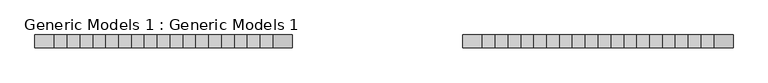
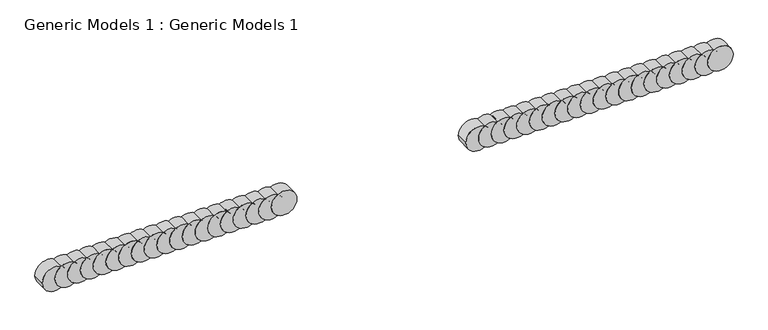
"""IFC4 building model written with IfcOpenShell, lengths in millimetres: proxy geometry, Generic Models 1 : Generic Models 1."""

from ifc_helpers import new_model, si_unit, point, frame, frame_2d, origin, place, context, project, spatial, circle_curve, trimmed, segment, composite_curve, outline, extrude, source, transform, mapped, element, save


def generic_models_1_generic_models_1_03ad02fd(model_context):
    return source(origin(), model_context, "Body", "SweptSolid", [
        extrude(outline(composite_curve([segment(trimmed(circle_curve(frame_2d((571.1323801, 6489.1161456)), 304.8), [point((571.1323801, 6184.3161456))], [point((571.1323801, 6793.9161456))], False, "CARTESIAN"), True, "CONTINUOUS"), segment(trimmed(circle_curve(frame_2d((571.1323801, 6489.1161456)), 304.8), [point((571.1323801, 6793.9161456))], [point((571.1323801, 6184.3161456))], False, "CARTESIAN"), True, "CONTINUOUS")], self_intersect=False)), frame((0.0, -13009.1052022, 0.0), z_axis=(0.0, 1.0, 0.0), x_axis=(0.0, 0.0, 1.0)), (0.0, 0.0, 1.0), 304.8),
        extrude(outline(composite_curve([segment(trimmed(circle_curve(frame_2d((571.1323801, 6184.3161456)), 304.8), [point((571.1323801, 5879.5161456))], [point((571.1323801, 6489.1161456))], False, "CARTESIAN"), True, "CONTINUOUS"), segment(trimmed(circle_curve(frame_2d((571.1323801, 6184.3161456)), 304.8), [point((571.1323801, 6489.1161456))], [point((571.1323801, 5879.5161456))], False, "CARTESIAN"), True, "CONTINUOUS")], self_intersect=False)), frame((0.0, -13009.1052022, 0.0), z_axis=(0.0, 1.0, 0.0), x_axis=(0.0, 0.0, 1.0)), (0.0, 0.0, 1.0), 304.8),
        extrude(outline(composite_curve([segment(trimmed(circle_curve(frame_2d((571.1323801, 5879.5161456)), 304.8), [point((571.1323801, 5574.7161456))], [point((571.1323801, 6184.3161456))], False, "CARTESIAN"), True, "CONTINUOUS"), segment(trimmed(circle_curve(frame_2d((571.1323801, 5879.5161456)), 304.8), [point((571.1323801, 6184.3161456))], [point((571.1323801, 5574.7161456))], False, "CARTESIAN"), True, "CONTINUOUS")], self_intersect=False)), frame((0.0, -13009.1052022, 0.0), z_axis=(0.0, 1.0, 0.0), x_axis=(0.0, 0.0, 1.0)), (0.0, 0.0, 1.0), 304.8),
        extrude(outline(composite_curve([segment(trimmed(circle_curve(frame_2d((571.1323801, 5574.7161456)), 304.8), [point((571.1323801, 5269.9161456))], [point((571.1323801, 5879.5161456))], False, "CARTESIAN"), True, "CONTINUOUS"), segment(trimmed(circle_curve(frame_2d((571.1323801, 5574.7161456)), 304.8), [point((571.1323801, 5879.5161456))], [point((571.1323801, 5269.9161456))], False, "CARTESIAN"), True, "CONTINUOUS")], self_intersect=False)), frame((0.0, -13009.1052022, 0.0), z_axis=(0.0, 1.0, 0.0), x_axis=(0.0, 0.0, 1.0)), (0.0, 0.0, 1.0), 304.8),
        extrude(outline(composite_curve([segment(trimmed(circle_curve(frame_2d((571.1323801, 5269.9161456)), 304.8), [point((571.1323801, 4965.1161456))], [point((571.1323801, 5574.7161456))], False, "CARTESIAN"), True, "CONTINUOUS"), segment(trimmed(circle_curve(frame_2d((571.1323801, 5269.9161456)), 304.8), [point((571.1323801, 5574.7161456))], [point((571.1323801, 4965.1161456))], False, "CARTESIAN"), True, "CONTINUOUS")], self_intersect=False)), frame((0.0, -13009.1052022, 0.0), z_axis=(0.0, 1.0, 0.0), x_axis=(0.0, 0.0, 1.0)), (0.0, 0.0, 1.0), 304.8),
        extrude(outline(composite_curve([segment(trimmed(circle_curve(frame_2d((571.1323801, 4965.1161456)), 304.8), [point((571.1323801, 4660.3161456))], [point((571.1323801, 5269.9161456))], False, "CARTESIAN"), True, "CONTINUOUS"), segment(trimmed(circle_curve(frame_2d((571.1323801, 4965.1161456)), 304.8), [point((571.1323801, 5269.9161456))], [point((571.1323801, 4660.3161456))], False, "CARTESIAN"), True, "CONTINUOUS")], self_intersect=False)), frame((0.0, -13009.1052022, 0.0), z_axis=(0.0, 1.0, 0.0), x_axis=(0.0, 0.0, 1.0)), (0.0, 0.0, 1.0), 304.8),
        extrude(outline(composite_curve([segment(trimmed(circle_curve(frame_2d((571.1323801, 4660.3161456)), 304.8), [point((571.1323801, 4355.5161456))], [point((571.1323801, 4965.1161456))], False, "CARTESIAN"), True, "CONTINUOUS"), segment(trimmed(circle_curve(frame_2d((571.1323801, 4660.3161456)), 304.8), [point((571.1323801, 4965.1161456))], [point((571.1323801, 4355.5161456))], False, "CARTESIAN"), True, "CONTINUOUS")], self_intersect=False)), frame((0.0, -13009.1052022, 0.0), z_axis=(0.0, 1.0, 0.0), x_axis=(0.0, 0.0, 1.0)), (0.0, 0.0, 1.0), 304.8),
        extrude(outline(composite_curve([segment(trimmed(circle_curve(frame_2d((571.1323801, 4355.5161456)), 304.8), [point((571.1323801, 4050.7161456))], [point((571.1323801, 4660.3161456))], False, "CARTESIAN"), True, "CONTINUOUS"), segment(trimmed(circle_curve(frame_2d((571.1323801, 4355.5161456)), 304.8), [point((571.1323801, 4660.3161456))], [point((571.1323801, 4050.7161456))], False, "CARTESIAN"), True, "CONTINUOUS")], self_intersect=False)), frame((0.0, -13009.1052022, 0.0), z_axis=(0.0, 1.0, 0.0), x_axis=(0.0, 0.0, 1.0)), (0.0, 0.0, 1.0), 304.8),
        extrude(outline(composite_curve([segment(trimmed(circle_curve(frame_2d((571.1323801, 4050.7161456)), 304.8), [point((571.1323801, 3745.9161456))], [point((571.1323801, 4355.5161456))], False, "CARTESIAN"), True, "CONTINUOUS"), segment(trimmed(circle_curve(frame_2d((571.1323801, 4050.7161456)), 304.8), [point((571.1323801, 4355.5161456))], [point((571.1323801, 3745.9161456))], False, "CARTESIAN"), True, "CONTINUOUS")], self_intersect=False)), frame((0.0, -13009.1052022, 0.0), z_axis=(0.0, 1.0, 0.0), x_axis=(0.0, 0.0, 1.0)), (0.0, 0.0, 1.0), 304.8),
        extrude(outline(composite_curve([segment(trimmed(circle_curve(frame_2d((571.1323801, 3745.9161456)), 304.8), [point((571.1323801, 3441.1161456))], [point((571.1323801, 4050.7161456))], False, "CARTESIAN"), True, "CONTINUOUS"), segment(trimmed(circle_curve(frame_2d((571.1323801, 3745.9161456)), 304.8), [point((571.1323801, 4050.7161456))], [point((571.1323801, 3441.1161456))], False, "CARTESIAN"), True, "CONTINUOUS")], self_intersect=False)), frame((0.0, -13009.1052022, 0.0), z_axis=(0.0, 1.0, 0.0), x_axis=(0.0, 0.0, 1.0)), (0.0, 0.0, 1.0), 304.8),
        extrude(outline(composite_curve([segment(trimmed(circle_curve(frame_2d((571.1323801, 3441.1161456)), 304.8), [point((571.1323801, 3136.3161456))], [point((571.1323801, 3745.9161456))], False, "CARTESIAN"), True, "CONTINUOUS"), segment(trimmed(circle_curve(frame_2d((571.1323801, 3441.1161456)), 304.8), [point((571.1323801, 3745.9161456))], [point((571.1323801, 3136.3161456))], False, "CARTESIAN"), True, "CONTINUOUS")], self_intersect=False)), frame((0.0, -13009.1052022, 0.0), z_axis=(0.0, 1.0, 0.0), x_axis=(0.0, 0.0, 1.0)), (0.0, 0.0, 1.0), 304.8),
        extrude(outline(composite_curve([segment(trimmed(circle_curve(frame_2d((571.1323801, 3136.3161456)), 304.8), [point((571.1323801, 2831.5161456))], [point((571.1323801, 3441.1161456))], False, "CARTESIAN"), True, "CONTINUOUS"), segment(trimmed(circle_curve(frame_2d((571.1323801, 3136.3161456)), 304.8), [point((571.1323801, 3441.1161456))], [point((571.1323801, 2831.5161456))], False, "CARTESIAN"), True, "CONTINUOUS")], self_intersect=False)), frame((0.0, -13009.1052022, 0.0), z_axis=(0.0, 1.0, 0.0), x_axis=(0.0, 0.0, 1.0)), (0.0, 0.0, 1.0), 304.8),
        extrude(outline(composite_curve([segment(trimmed(circle_curve(frame_2d((571.1323801, 2831.5161456)), 304.8), [point((571.1323801, 2526.7161456))], [point((571.1323801, 3136.3161456))], False, "CARTESIAN"), True, "CONTINUOUS"), segment(trimmed(circle_curve(frame_2d((571.1323801, 2831.5161456)), 304.8), [point((571.1323801, 3136.3161456))], [point((571.1323801, 2526.7161456))], False, "CARTESIAN"), True, "CONTINUOUS")], self_intersect=False)), frame((0.0, -13009.1052022, 0.0), z_axis=(0.0, 1.0, 0.0), x_axis=(0.0, 0.0, 1.0)), (0.0, 0.0, 1.0), 304.8),
        extrude(outline(composite_curve([segment(trimmed(circle_curve(frame_2d((571.1323801, 2526.7161456)), 304.8), [point((571.1323801, 2221.9161456))], [point((571.1323801, 2831.5161456))], False, "CARTESIAN"), True, "CONTINUOUS"), segment(trimmed(circle_curve(frame_2d((571.1323801, 2526.7161456)), 304.8), [point((571.1323801, 2831.5161456))], [point((571.1323801, 2221.9161456))], False, "CARTESIAN"), True, "CONTINUOUS")], self_intersect=False)), frame((0.0, -13009.1052022, 0.0), z_axis=(0.0, 1.0, 0.0), x_axis=(0.0, 0.0, 1.0)), (0.0, 0.0, 1.0), 304.8),
        extrude(outline(composite_curve([segment(trimmed(circle_curve(frame_2d((571.1323801, 2221.9161456)), 304.8), [point((571.1323801, 1917.1161456))], [point((571.1323801, 2526.7161456))], False, "CARTESIAN"), True, "CONTINUOUS"), segment(trimmed(circle_curve(frame_2d((571.1323801, 2221.9161456)), 304.8), [point((571.1323801, 2526.7161456))], [point((571.1323801, 1917.1161456))], False, "CARTESIAN"), True, "CONTINUOUS")], self_intersect=False)), frame((0.0, -13009.1052022, 0.0), z_axis=(0.0, 1.0, 0.0), x_axis=(0.0, 0.0, 1.0)), (0.0, 0.0, 1.0), 304.8),
        extrude(outline(composite_curve([segment(trimmed(circle_curve(frame_2d((571.1323801, 1917.1161456)), 304.8), [point((571.1323801, 1612.3161456))], [point((571.1323801, 2221.9161456))], False, "CARTESIAN"), True, "CONTINUOUS"), segment(trimmed(circle_curve(frame_2d((571.1323801, 1917.1161456)), 304.8), [point((571.1323801, 2221.9161456))], [point((571.1323801, 1612.3161456))], False, "CARTESIAN"), True, "CONTINUOUS")], self_intersect=False)), frame((0.0, -13009.1052022, 0.0), z_axis=(0.0, 1.0, 0.0), x_axis=(0.0, 0.0, 1.0)), (0.0, 0.0, 1.0), 304.8),
        extrude(outline(composite_curve([segment(trimmed(circle_curve(frame_2d((571.1323801, 1612.3161456)), 304.8), [point((571.1323801, 1307.5161456))], [point((571.1323801, 1917.1161456))], False, "CARTESIAN"), True, "CONTINUOUS"), segment(trimmed(circle_curve(frame_2d((571.1323801, 1612.3161456)), 304.8), [point((571.1323801, 1917.1161456))], [point((571.1323801, 1307.5161456))], False, "CARTESIAN"), True, "CONTINUOUS")], self_intersect=False)), frame((0.0, -13009.1052022, 0.0), z_axis=(0.0, 1.0, 0.0), x_axis=(0.0, 0.0, 1.0)), (0.0, 0.0, 1.0), 304.8),
        extrude(outline(composite_curve([segment(trimmed(circle_curve(frame_2d((571.1323801, 1307.5161456)), 304.8), [point((571.1323801, 1002.7161456))], [point((571.1323801, 1612.3161456))], False, "CARTESIAN"), True, "CONTINUOUS"), segment(trimmed(circle_curve(frame_2d((571.1323801, 1307.5161456)), 304.8), [point((571.1323801, 1612.3161456))], [point((571.1323801, 1002.7161456))], False, "CARTESIAN"), True, "CONTINUOUS")], self_intersect=False)), frame((0.0, -13009.1052022, 0.0), z_axis=(0.0, 1.0, 0.0), x_axis=(0.0, 0.0, 1.0)), (0.0, 0.0, 1.0), 304.8),
        extrude(outline(composite_curve([segment(trimmed(circle_curve(frame_2d((571.1323801, 1002.7161456)), 304.8), [point((571.1323801, 697.9161456))], [point((571.1323801, 1307.5161456))], False, "CARTESIAN"), True, "CONTINUOUS"), segment(trimmed(circle_curve(frame_2d((571.1323801, 1002.7161456)), 304.8), [point((571.1323801, 1307.5161456))], [point((571.1323801, 697.9161456))], False, "CARTESIAN"), True, "CONTINUOUS")], self_intersect=False)), frame((0.0, -13009.1052022, 0.0), z_axis=(0.0, 1.0, 0.0), x_axis=(0.0, 0.0, 1.0)), (0.0, 0.0, 1.0), 304.8),
        extrude(outline(composite_curve([segment(trimmed(circle_curve(frame_2d((571.1323801, 697.9161456)), 304.8), [point((571.1323801, 393.1161456))], [point((571.1323801, 1002.7161456))], False, "CARTESIAN"), True, "CONTINUOUS"), segment(trimmed(circle_curve(frame_2d((571.1323801, 697.9161456)), 304.8), [point((571.1323801, 1002.7161456))], [point((571.1323801, 393.1161456))], False, "CARTESIAN"), True, "CONTINUOUS")], self_intersect=False)), frame((0.0, -13009.1052022, 0.0), z_axis=(0.0, 1.0, 0.0), x_axis=(0.0, 0.0, 1.0)), (0.0, 0.0, 1.0), 304.8),
        extrude(outline(composite_curve([segment(trimmed(circle_curve(frame_2d((571.1323801, -3957.3992242)), 304.8), [point((571.1323801, -4262.1992242))], [point((571.1323801, -3652.5992242))], False, "CARTESIAN"), True, "CONTINUOUS"), segment(trimmed(circle_curve(frame_2d((571.1323801, -3957.3992242)), 304.8), [point((571.1323801, -3652.5992242))], [point((571.1323801, -4262.1992242))], False, "CARTESIAN"), True, "CONTINUOUS")], self_intersect=False)), frame((0.0, -13009.1052022, 0.0), z_axis=(0.0, 1.0, 0.0), x_axis=(0.0, 0.0, 1.0)), (0.0, 0.0, 1.0), 304.8),
        extrude(outline(composite_curve([segment(trimmed(circle_curve(frame_2d((571.1323801, -4262.1992242)), 304.8), [point((571.1323801, -4566.9992242))], [point((571.1323801, -3957.3992242))], False, "CARTESIAN"), True, "CONTINUOUS"), segment(trimmed(circle_curve(frame_2d((571.1323801, -4262.1992242)), 304.8), [point((571.1323801, -3957.3992242))], [point((571.1323801, -4566.9992242))], False, "CARTESIAN"), True, "CONTINUOUS")], self_intersect=False)), frame((0.0, -13009.1052022, 0.0), z_axis=(0.0, 1.0, 0.0), x_axis=(0.0, 0.0, 1.0)), (0.0, 0.0, 1.0), 304.8),
        extrude(outline(composite_curve([segment(trimmed(circle_curve(frame_2d((571.1323801, -4566.9992242)), 304.8), [point((571.1323801, -4871.7992242))], [point((571.1323801, -4262.1992242))], False, "CARTESIAN"), True, "CONTINUOUS"), segment(trimmed(circle_curve(frame_2d((571.1323801, -4566.9992242)), 304.8), [point((571.1323801, -4262.1992242))], [point((571.1323801, -4871.7992242))], False, "CARTESIAN"), True, "CONTINUOUS")], self_intersect=False)), frame((0.0, -13009.1052022, 0.0), z_axis=(0.0, 1.0, 0.0), x_axis=(0.0, 0.0, 1.0)), (0.0, 0.0, 1.0), 304.8),
        extrude(outline(composite_curve([segment(trimmed(circle_curve(frame_2d((571.1323801, -4871.7992242)), 304.8), [point((571.1323801, -5176.5992242))], [point((571.1323801, -4566.9992242))], False, "CARTESIAN"), True, "CONTINUOUS"), segment(trimmed(circle_curve(frame_2d((571.1323801, -4871.7992242)), 304.8), [point((571.1323801, -4566.9992242))], [point((571.1323801, -5176.5992242))], False, "CARTESIAN"), True, "CONTINUOUS")], self_intersect=False)), frame((0.0, -13009.1052022, 0.0), z_axis=(0.0, 1.0, 0.0), x_axis=(0.0, 0.0, 1.0)), (0.0, 0.0, 1.0), 304.8),
        extrude(outline(composite_curve([segment(trimmed(circle_curve(frame_2d((571.1323801, -5176.5992242)), 304.8), [point((571.1323801, -5481.3992242))], [point((571.1323801, -4871.7992242))], False, "CARTESIAN"), True, "CONTINUOUS"), segment(trimmed(circle_curve(frame_2d((571.1323801, -5176.5992242)), 304.8), [point((571.1323801, -4871.7992242))], [point((571.1323801, -5481.3992242))], False, "CARTESIAN"), True, "CONTINUOUS")], self_intersect=False)), frame((0.0, -13009.1052022, 0.0), z_axis=(0.0, 1.0, 0.0), x_axis=(0.0, 0.0, 1.0)), (0.0, 0.0, 1.0), 304.8),
        extrude(outline(composite_curve([segment(trimmed(circle_curve(frame_2d((571.1323801, -5481.3992242)), 304.8), [point((571.1323801, -5786.1992242))], [point((571.1323801, -5176.5992242))], False, "CARTESIAN"), True, "CONTINUOUS"), segment(trimmed(circle_curve(frame_2d((571.1323801, -5481.3992242)), 304.8), [point((571.1323801, -5176.5992242))], [point((571.1323801, -5786.1992242))], False, "CARTESIAN"), True, "CONTINUOUS")], self_intersect=False)), frame((0.0, -13009.1052022, 0.0), z_axis=(0.0, 1.0, 0.0), x_axis=(0.0, 0.0, 1.0)), (0.0, 0.0, 1.0), 304.8),
        extrude(outline(composite_curve([segment(trimmed(circle_curve(frame_2d((571.1323801, -5786.1992242)), 304.8), [point((571.1323801, -6090.9992242))], [point((571.1323801, -5481.3992242))], False, "CARTESIAN"), True, "CONTINUOUS"), segment(trimmed(circle_curve(frame_2d((571.1323801, -5786.1992242)), 304.8), [point((571.1323801, -5481.3992242))], [point((571.1323801, -6090.9992242))], False, "CARTESIAN"), True, "CONTINUOUS")], self_intersect=False)), frame((0.0, -13009.1052022, 0.0), z_axis=(0.0, 1.0, 0.0), x_axis=(0.0, 0.0, 1.0)), (0.0, 0.0, 1.0), 304.8),
        extrude(outline(composite_curve([segment(trimmed(circle_curve(frame_2d((571.1323801, -6090.9992242)), 304.8), [point((571.1323801, -6395.7992242))], [point((571.1323801, -5786.1992242))], False, "CARTESIAN"), True, "CONTINUOUS"), segment(trimmed(circle_curve(frame_2d((571.1323801, -6090.9992242)), 304.8), [point((571.1323801, -5786.1992242))], [point((571.1323801, -6395.7992242))], False, "CARTESIAN"), True, "CONTINUOUS")], self_intersect=False)), frame((0.0, -13009.1052022, 0.0), z_axis=(0.0, 1.0, 0.0), x_axis=(0.0, 0.0, 1.0)), (0.0, 0.0, 1.0), 304.8),
        extrude(outline(composite_curve([segment(trimmed(circle_curve(frame_2d((571.1323801, -6395.7992242)), 304.8), [point((571.1323801, -6700.5992242))], [point((571.1323801, -6090.9992242))], False, "CARTESIAN"), True, "CONTINUOUS"), segment(trimmed(circle_curve(frame_2d((571.1323801, -6395.7992242)), 304.8), [point((571.1323801, -6090.9992242))], [point((571.1323801, -6700.5992242))], False, "CARTESIAN"), True, "CONTINUOUS")], self_intersect=False)), frame((0.0, -13009.1052022, 0.0), z_axis=(0.0, 1.0, 0.0), x_axis=(0.0, 0.0, 1.0)), (0.0, 0.0, 1.0), 304.8),
        extrude(outline(composite_curve([segment(trimmed(circle_curve(frame_2d((571.1323801, -6700.5992242)), 304.8), [point((571.1323801, -7005.3992242))], [point((571.1323801, -6395.7992242))], False, "CARTESIAN"), True, "CONTINUOUS"), segment(trimmed(circle_curve(frame_2d((571.1323801, -6700.5992242)), 304.8), [point((571.1323801, -6395.7992242))], [point((571.1323801, -7005.3992242))], False, "CARTESIAN"), True, "CONTINUOUS")], self_intersect=False)), frame((0.0, -13009.1052022, 0.0), z_axis=(0.0, 1.0, 0.0), x_axis=(0.0, 0.0, 1.0)), (0.0, 0.0, 1.0), 304.8),
        extrude(outline(composite_curve([segment(trimmed(circle_curve(frame_2d((571.1323801, -7005.3992242)), 304.8), [point((571.1323801, -7310.1992242))], [point((571.1323801, -6700.5992242))], False, "CARTESIAN"), True, "CONTINUOUS"), segment(trimmed(circle_curve(frame_2d((571.1323801, -7005.3992242)), 304.8), [point((571.1323801, -6700.5992242))], [point((571.1323801, -7310.1992242))], False, "CARTESIAN"), True, "CONTINUOUS")], self_intersect=False)), frame((0.0, -13009.1052022, 0.0), z_axis=(0.0, 1.0, 0.0), x_axis=(0.0, 0.0, 1.0)), (0.0, 0.0, 1.0), 304.8),
        extrude(outline(composite_curve([segment(trimmed(circle_curve(frame_2d((571.1323801, -7310.1992242)), 304.8), [point((571.1323801, -7614.9992242))], [point((571.1323801, -7005.3992242))], False, "CARTESIAN"), True, "CONTINUOUS"), segment(trimmed(circle_curve(frame_2d((571.1323801, -7310.1992242)), 304.8), [point((571.1323801, -7005.3992242))], [point((571.1323801, -7614.9992242))], False, "CARTESIAN"), True, "CONTINUOUS")], self_intersect=False)), frame((0.0, -13009.1052022, 0.0), z_axis=(0.0, 1.0, 0.0), x_axis=(0.0, 0.0, 1.0)), (0.0, 0.0, 1.0), 304.8),
        extrude(outline(composite_curve([segment(trimmed(circle_curve(frame_2d((571.1323801, -7614.9992242)), 304.8), [point((571.1323801, -7919.7992242))], [point((571.1323801, -7310.1992242))], False, "CARTESIAN"), True, "CONTINUOUS"), segment(trimmed(circle_curve(frame_2d((571.1323801, -7614.9992242)), 304.8), [point((571.1323801, -7310.1992242))], [point((571.1323801, -7919.7992242))], False, "CARTESIAN"), True, "CONTINUOUS")], self_intersect=False)), frame((0.0, -13009.1052022, 0.0), z_axis=(0.0, 1.0, 0.0), x_axis=(0.0, 0.0, 1.0)), (0.0, 0.0, 1.0), 304.8),
        extrude(outline(composite_curve([segment(trimmed(circle_curve(frame_2d((571.1323801, -7919.7992242)), 304.8), [point((571.1323801, -8224.5992242))], [point((571.1323801, -7614.9992242))], False, "CARTESIAN"), True, "CONTINUOUS"), segment(trimmed(circle_curve(frame_2d((571.1323801, -7919.7992242)), 304.8), [point((571.1323801, -7614.9992242))], [point((571.1323801, -8224.5992242))], False, "CARTESIAN"), True, "CONTINUOUS")], self_intersect=False)), frame((0.0, -13009.1052022, 0.0), z_axis=(0.0, 1.0, 0.0), x_axis=(0.0, 0.0, 1.0)), (0.0, 0.0, 1.0), 304.8),
        extrude(outline(composite_curve([segment(trimmed(circle_curve(frame_2d((571.1323801, -8224.5992242)), 304.8), [point((571.1323801, -8529.3992242))], [point((571.1323801, -7919.7992242))], False, "CARTESIAN"), True, "CONTINUOUS"), segment(trimmed(circle_curve(frame_2d((571.1323801, -8224.5992242)), 304.8), [point((571.1323801, -7919.7992242))], [point((571.1323801, -8529.3992242))], False, "CARTESIAN"), True, "CONTINUOUS")], self_intersect=False)), frame((0.0, -13009.1052022, 0.0), z_axis=(0.0, 1.0, 0.0), x_axis=(0.0, 0.0, 1.0)), (0.0, 0.0, 1.0), 304.8),
        extrude(outline(composite_curve([segment(trimmed(circle_curve(frame_2d((571.1323801, -8529.3992242)), 304.8), [point((571.1323801, -8834.1992242))], [point((571.1323801, -8224.5992242))], False, "CARTESIAN"), True, "CONTINUOUS"), segment(trimmed(circle_curve(frame_2d((571.1323801, -8529.3992242)), 304.8), [point((571.1323801, -8224.5992242))], [point((571.1323801, -8834.1992242))], False, "CARTESIAN"), True, "CONTINUOUS")], self_intersect=False)), frame((0.0, -13009.1052022, 0.0), z_axis=(0.0, 1.0, 0.0), x_axis=(0.0, 0.0, 1.0)), (0.0, 0.0, 1.0), 304.8),
        extrude(outline(composite_curve([segment(trimmed(circle_curve(frame_2d((571.1323801, -8834.1992242)), 304.8), [point((571.1323801, -9138.9992242))], [point((571.1323801, -8529.3992242))], False, "CARTESIAN"), True, "CONTINUOUS"), segment(trimmed(circle_curve(frame_2d((571.1323801, -8834.1992242)), 304.8), [point((571.1323801, -8529.3992242))], [point((571.1323801, -9138.9992242))], False, "CARTESIAN"), True, "CONTINUOUS")], self_intersect=False)), frame((0.0, -13009.1052022, 0.0), z_axis=(0.0, 1.0, 0.0), x_axis=(0.0, 0.0, 1.0)), (0.0, 0.0, 1.0), 304.8),
        extrude(outline(composite_curve([segment(trimmed(circle_curve(frame_2d((571.1323801, -9138.9992242)), 304.8), [point((571.1323801, -9443.7992242))], [point((571.1323801, -8834.1992242))], False, "CARTESIAN"), True, "CONTINUOUS"), segment(trimmed(circle_curve(frame_2d((571.1323801, -9138.9992242)), 304.8), [point((571.1323801, -8834.1992242))], [point((571.1323801, -9443.7992242))], False, "CARTESIAN"), True, "CONTINUOUS")], self_intersect=False)), frame((0.0, -13009.1052022, 0.0), z_axis=(0.0, 1.0, 0.0), x_axis=(0.0, 0.0, 1.0)), (0.0, 0.0, 1.0), 304.8),
        extrude(outline(composite_curve([segment(trimmed(circle_curve(frame_2d((571.1323801, -9443.7992242)), 304.8), [point((571.1323801, -9748.5992242))], [point((571.1323801, -9138.9992242))], False, "CARTESIAN"), True, "CONTINUOUS"), segment(trimmed(circle_curve(frame_2d((571.1323801, -9443.7992242)), 304.8), [point((571.1323801, -9138.9992242))], [point((571.1323801, -9748.5992242))], False, "CARTESIAN"), True, "CONTINUOUS")], self_intersect=False)), frame((0.0, -13009.1052022, 0.0), z_axis=(0.0, 1.0, 0.0), x_axis=(0.0, 0.0, 1.0)), (0.0, 0.0, 1.0), 304.8),
    ])


if __name__ == "__main__":
    model = new_model("IFC4")
    model_context = context("Model", 3, world=origin())
    ifc_project = project(units=[si_unit("LENGTHUNIT", "METRE", prefix="MILLI")], contexts=[model_context])
    site = spatial("IfcSite", under=ifc_project)
    building = spatial("IfcBuilding", under=site)
    placement = place(None, origin())
    generic_models_1_generic_models_1_shape = generic_models_1_generic_models_1_03ad02fd(model_context)
    element("IfcBuildingElementProxy", 1, Name="Generic Models 1 : Generic Models 1", ObjectType="Generic Models 1 : Generic Models 1", at=placement, inside=building, context=model_context, shape_type="MappedRepresentation", body=[
        mapped(generic_models_1_generic_models_1_shape, transform((0.0, 0.0, 0.0), x_axis=(1.0, 0.0, 0.0), y_axis=(0.0, 1.0, 0.0), z_axis=(0.0, 0.0, 1.0))),
    ])
    save(model, "model.ifc")

# Revit data of these elements
# Element 1 (IfcBuildingElementProxy, "Generic Models 1 : Generic Models 1")
#   Materials on its faces: "Brick, Soldier Course"
# Materials
#   "Brick, Soldier Course": class "Masonry", colour RGB 170 98 104, transparency 0, Description = "Common brick soldier coursed", Cost = 0
